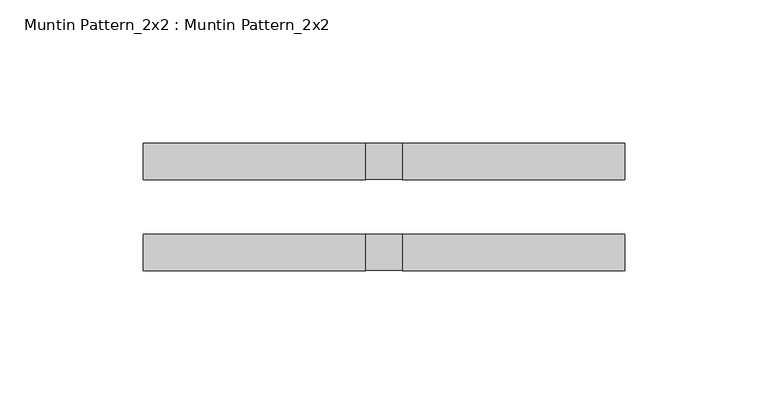
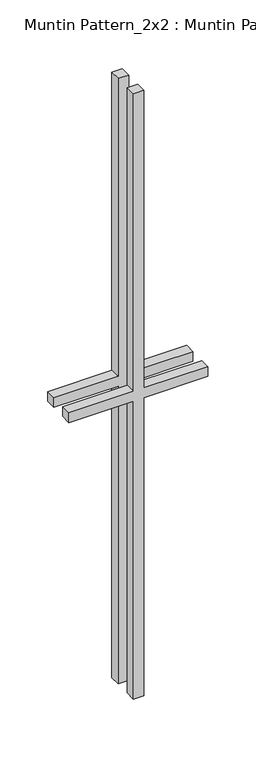
"""IFC4 building model written with IfcOpenShell, lengths in millimetres: proxy geometry, Muntin Pattern_2x2 : Muntin Pattern_2x2."""

from ifc_helpers import new_model, si_unit, frame, origin, place, context, project, spatial, polyline, outline, extrude, source, transform, mapped, element, save


def muntin_pattern_2x2_muntin_pattern_2x2_e8f3e573(model_context):
    return source(origin(), model_context, "Body", "SweptSolid", [
        extrude(outline(polyline([(393.7, -6.35), (393.7, -84.1375), (381.0, -84.1375), (381.0, -6.35), (0.0, -6.35), (0.0, 6.35), (381.0, 6.35), (381.0, 84.1375), (393.7, 84.1375), (393.7, 6.35), (774.7, 6.35), (774.7, -6.35), (393.7, -6.35)])), frame((0.0, -22.225, 0.0), z_axis=(0.0, 1.0, 0.0), x_axis=(0.0, 0.0, 1.0)), (0.0, 0.0, 1.0), 12.7),
        extrude(outline(polyline([(393.7, -6.35), (393.7, -84.1375), (381.0, -84.1375), (381.0, -6.35), (0.0, -6.35), (0.0, 6.35), (381.0, 6.35), (381.0, 84.1375), (393.7, 84.1375), (393.7, 6.35), (774.7, 6.35), (774.7, -6.35), (393.7, -6.35)])), frame((0.0, 9.525, 0.0), z_axis=(0.0, 1.0, 0.0), x_axis=(0.0, 0.0, 1.0)), (0.0, 0.0, 1.0), 12.7),
    ])


if __name__ == "__main__":
    model = new_model("IFC4")
    model_context = context("Model", 3, world=origin())
    ifc_project = project(units=[si_unit("LENGTHUNIT", "METRE", prefix="MILLI")], contexts=[model_context])
    site = spatial("IfcSite", under=ifc_project)
    building = spatial("IfcBuilding", under=site)
    placement = place(None, origin())
    muntin_pattern_2x2_muntin_pattern_2x2_shape = muntin_pattern_2x2_muntin_pattern_2x2_e8f3e573(model_context)
    element("IfcBuildingElementProxy", 1, Name="Muntin Pattern_2x2 : Muntin Pattern_2x2", ObjectType="Muntin Pattern_2x2 : Muntin Pattern_2x2", at=placement, inside=building, context=model_context, shape_type="MappedRepresentation", body=[
        mapped(muntin_pattern_2x2_muntin_pattern_2x2_shape, transform((0.0, 0.0, 0.0), x_axis=(1.0, 0.0, 0.0), y_axis=(0.0, 1.0, 0.0), z_axis=(0.0, 0.0, 1.0))),
    ])
    save(model, "model.ifc")

# Revit data of these elements
# Type "Muntin Pattern_2x2 : Muntin Pattern_2x2"
#   Width [instance default] = 4' - 0"
#   Thickness = 0' - 0 1/2"
#   Height [instance default] = 4' - 0"
#   Distance = 0' - 0 3/4"
#   Interior Material [instance default] = none
#   Exterior Material [instance default] = none
#   Default Elevation = 0
# Element 1 (IfcBuildingElementProxy, "Muntin Pattern_2x2 : Muntin Pattern_2x2")
#   Width = 0' - 6 5/8"
#   Height = 2' - 6 1/2"
#   Interior Material = Wood - Stained
#   Exterior Material = Clad - White
#   Materials on its faces: "Clad - White", "Wood - Stained"
# Materials
#   "Clad - White": class "Wood", colour RGB 242 242 238, transparency 0, Cost = 0
#   "Wood - Stained": class "Wood", colour RGB 224 178 126, transparency 0, Cost = 0
